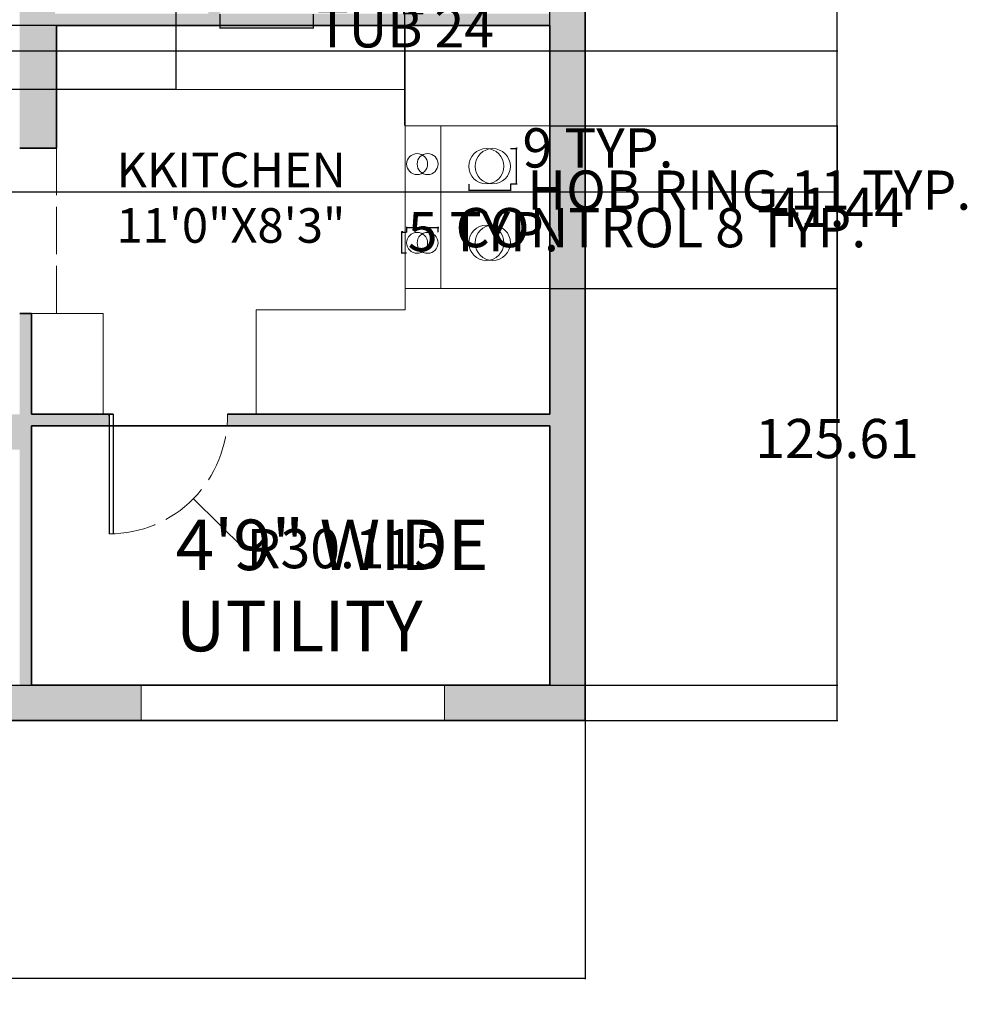
# Model space of a CAD drawing. Units: inches. Extents: x 300 to 1007, y 2 to 1069.
# Tile 6 of 12: x 766 to 1007, y 2 to 253. Entities that reach past the tile are written whole.
import ezdxf

# ---------------------------------------------------------------- set-up
doc = ezdxf.new("R2010")
doc.units = ezdxf.units.IN
doc.header["$MEASUREMENT"] = 0
doc.linetypes.add('ACAD_ISO02W100', pattern=[15, 12, -3])
for name, color, linetype, lineweight in [('A-ANNO-DIMS', 2, 'Continuous', 18), ('A-AREA-IDEN', 7, 'Continuous', 18), ('A-CASE', 8, 'Continuous', 18), ('A-DOOR', 3, 'Continuous', 25), ('A-DOOR-SWNG', 3, 'ACAD_ISO02W100', 13), ('A-EQPM', 9, 'Continuous', 18), ('A-GLAZ', 4, 'Continuous', 18), ('A-WALL', 7, 'Continuous', 35), ('A-WALL-OVHD', 8, 'ACAD_ISO02W100', 18)]:
    doc.layers.add(name, color=color, linetype=linetype, lineweight=lineweight)
doc.layers.add('A-WALL-PATT', color=9, linetype='Continuous', lineweight=9, true_color=0xc7c8ca)
doc.styles.get("Standard").update_dxf_attribs({"font": 'arial.ttf'})
doc.dimstyles.get("Standard").update_dxf_attribs({"dimtxt": 10, "dimasz": 0.18, "dimexe": 0.18, "dimexo": 0.0625, "dimgap": 0.09, "dimtad": 0, "dimtih": 1, "dimtoh": 1, "dimdec": 0, "dimzin": 0, "dimdsep": 46, "dimlunit": 3, "dimtxsty": 'Standard', "dimcen": 0.09, "dimadec": 0, "dimazin": 0, "dimtfac": 1, "dimtdec": 0, "dimtofl": 0, "dimtmove": 0, "dimatfit": 3, "dimfxl": 1, "dimtolj": 1, "dimtzin": 0, "dimarcsym": 0})

# ---------------------------------------------------------------- blocks, each defined once
blk = doc.blocks.new('COOKTOP-RING-9')
for centre in [(0, 0), (1.63, 0)]:
    blk.add_circle(centre, 4.49)
blk = doc.blocks.new('COOKTOP-CONTROL-5')
for centre in [(0, 0), (2.67, 0)]:
    blk.add_circle(centre, 2.67)
blk = doc.blocks.new('*D31')
at = {"layer": 'A-ANNO-DIMS', "color": 0, "lineweight": -2, "transparency": 16777216}
for p, q in [((868.84, 287.43), (863.76, 287.43)), ((863.94, 287.25), (863.94, 276.17)), ((863.94, 254.56), (863.94, 265.64)), ((868.84, 254.38), (863.76, 254.38))]:
    blk.add_line(p, q, dxfattribs=at)
at = {"layer": 'A-ANNO-DIMS', "color": 0, "transparency": 16777216}
for points in [[(863.91, 287.25), (863.97, 287.25), (863.94, 287.43)], [(863.91, 254.56), (863.97, 254.56), (863.94, 254.38)]]:
    blk.add_solid(points, dxfattribs=at)
at = {"layer": 'Defpoints', "color": 0, "transparency": 16777216}
for p in [(868.9, 287.43), (863.94, 254.38), (868.9, 254.38)]:
    blk.add_point(p, dxfattribs=at)
at = {"layer": 'A-ANNO-DIMS', "color": 0, "transparency": 16777216, "insert": (863.94, 270.91), "char_height": 10, "attachment_point": 5}
blk.add_mtext('\\A1;WC 33 TYP.', dxfattribs=at)
blk = doc.blocks.new('*D37')
at = {"layer": 'A-ANNO-DIMS', "color": 0, "lineweight": -2, "transparency": 16777216}
for p, q in [((817.12, 254.32), (817.12, 250.64)), ((840.87, 254.32), (840.87, 250.64)), ((817.3, 250.82), (840.69, 250.82)), ((840.87, 250.82), (841.05, 250.82))]:
    blk.add_line(p, q, dxfattribs=at)
at = {"layer": 'A-ANNO-DIMS', "color": 0, "transparency": 16777216}
for points in [[(817.3, 250.85), (817.3, 250.79), (817.12, 250.82)], [(840.69, 250.85), (840.69, 250.79), (840.87, 250.82)]]:
    blk.add_solid(points, dxfattribs=at)
at = {"layer": 'Defpoints', "color": 0, "transparency": 16777216}
for p in [(817.12, 254.38), (840.87, 254.38), (840.87, 250.82)]:
    blk.add_point(p, dxfattribs=at)
at = {"layer": 'A-ANNO-DIMS', "color": 0, "transparency": 16777216, "insert": (864.32, 250.82), "char_height": 10, "attachment_point": 5}
blk.add_mtext('\\A1;TUB 24', dxfattribs=at)
blk = doc.blocks.new('*D67')
at = {"layer": 'A-ANNO-DIMS', "color": 0, "lineweight": -2, "transparency": 16777216}
for p, q in [((880.48, 211), (880.48, 209.29)), ((891.09, 211), (891.09, 209.29)), ((880.66, 209.47), (890.91, 209.47)), ((891.09, 209.47), (891.27, 209.47))]:
    blk.add_line(p, q, dxfattribs=at)
at = {"layer": 'A-ANNO-DIMS', "color": 0, "transparency": 16777216}
for points in [[(880.66, 209.5), (880.66, 209.44), (880.48, 209.47)], [(890.91, 209.5), (890.91, 209.44), (891.09, 209.47)]]:
    blk.add_solid(points, dxfattribs=at)
at = {"layer": 'Defpoints', "color": 0, "transparency": 16777216}
for p in [(880.48, 211.06), (891.09, 211.06), (891.09, 209.47)]:
    blk.add_point(p, dxfattribs=at)
at = {"layer": 'A-ANNO-DIMS', "color": 0, "transparency": 16777216, "insert": (951.91, 209.47), "char_height": 10, "attachment_point": 5}
blk.add_mtext('\\A1;HOB RING 11 TYP.', dxfattribs=at)
blk = doc.blocks.new('*D68')
at = {"layer": 'A-ANNO-DIMS', "color": 0, "lineweight": -2, "transparency": 16777216}
for p, q in [((891.15, 220.04), (892.86, 220.04)), ((892.68, 220.04), (892.68, 220.22)), ((892.68, 220.22), (892.86, 220.22)), ((892.68, 211.24), (892.68, 219.86)), ((891.15, 211.06), (892.86, 211.06))]:
    blk.add_line(p, q, dxfattribs=at)
at = {"layer": 'A-ANNO-DIMS', "color": 0, "transparency": 16777216}
for points in [[(892.65, 219.86), (892.71, 219.86), (892.68, 220.04)], [(892.65, 211.24), (892.71, 211.24), (892.68, 211.06)]]:
    blk.add_solid(points, dxfattribs=at)
at = {"layer": 'Defpoints', "color": 0, "transparency": 16777216}
for p in [(891.09, 220.04), (892.68, 220.04), (891.09, 211.06)]:
    blk.add_point(p, dxfattribs=at)
at = {"layer": 'A-ANNO-DIMS', "color": 0, "transparency": 16777216, "insert": (913.4, 220.22), "char_height": 10, "attachment_point": 5}
blk.add_mtext('\\A1;9 TYP.', dxfattribs=at)
blk = doc.blocks.new('*D69')
at = {"layer": 'A-ANNO-DIMS', "color": 0, "lineweight": -2, "transparency": 16777216}
for p, q in [((864.68, 198.77), (864.68, 200.09)), ((864.86, 199.91), (872.49, 199.91)), ((872.67, 198.77), (872.67, 200.09)), ((872.67, 199.91), (872.85, 199.91))]:
    blk.add_line(p, q, dxfattribs=at)
at = {"layer": 'A-ANNO-DIMS', "color": 0, "transparency": 16777216}
for points in [[(864.86, 199.94), (864.86, 199.88), (864.68, 199.91)], [(872.49, 199.94), (872.49, 199.88), (872.67, 199.91)]]:
    blk.add_solid(points, dxfattribs=at)
at = {"layer": 'Defpoints', "color": 0, "transparency": 16777216}
for p in [(864.68, 198.71), (872.67, 199.91), (872.67, 198.71)]:
    blk.add_point(p, dxfattribs=at)
at = {"layer": 'A-ANNO-DIMS', "color": 0, "transparency": 16777216, "insert": (929.43, 199.91), "char_height": 10, "attachment_point": 5}
blk.add_mtext('\\A1;CONTROL 8 TYP.', dxfattribs=at)
blk = doc.blocks.new('*D70')
at = {"layer": 'A-ANNO-DIMS', "color": 0, "lineweight": -2, "transparency": 16777216}
for p, q in [((864.61, 198.71), (863.3, 198.71)), ((863.48, 198.71), (863.48, 198.89)), ((863.48, 198.89), (863.66, 198.89)), ((863.48, 193.56), (863.48, 198.53)), ((864.61, 193.38), (863.3, 193.38))]:
    blk.add_line(p, q, dxfattribs=at)
at = {"layer": 'A-ANNO-DIMS', "color": 0, "transparency": 16777216}
for points in [[(863.45, 198.53), (863.51, 198.53), (863.48, 198.71)], [(863.45, 193.56), (863.51, 193.56), (863.48, 193.38)]]:
    blk.add_solid(points, dxfattribs=at)
at = {"layer": 'Defpoints', "color": 0, "transparency": 16777216}
for p in [(863.48, 198.71), (864.68, 198.71), (864.68, 193.38)]:
    blk.add_point(p, dxfattribs=at)
at = {"layer": 'A-ANNO-DIMS', "color": 0, "transparency": 16777216, "insert": (884.2, 198.89), "char_height": 10, "attachment_point": 5}
blk.add_mtext('\\A1;5 TYP.', dxfattribs=at)
blk = doc.blocks.new('*D73')
at = {"layer": 'A-ANNO-DIMS', "color": 0, "lineweight": -2, "transparency": 16777216}
for p, q in [((420.12, 74.32), (420.12, 8.45)), ((910.12, 74.32), (910.12, 8.45)), ((420.3, 8.63), (653.8, 8.63)), ((909.94, 8.63), (676.44, 8.63))]:
    blk.add_line(p, q, dxfattribs=at)
at = {"layer": 'A-ANNO-DIMS', "color": 0, "transparency": 16777216}
for points in [[(420.3, 8.66), (420.3, 8.6), (420.12, 8.63)], [(909.94, 8.66), (909.94, 8.6), (910.12, 8.63)]]:
    blk.add_solid(points, dxfattribs=at)
at = {"layer": 'Defpoints', "color": 0, "transparency": 16777216}
for p in [(420.12, 74.38), (910.12, 74.38), (910.12, 8.63)]:
    blk.add_point(p, dxfattribs=at)
at = {"layer": 'A-ANNO-DIMS', "color": 0, "transparency": 16777216, "insert": (665.12, 8.63), "char_height": 10, "attachment_point": 5}
blk.add_mtext('\\A1;490', dxfattribs=at)
blk = doc.blocks.new('*D76')
at = {"layer": 'A-ANNO-DIMS', "color": 0, "lineweight": -2, "transparency": 16777216}
for p, q in [((910.18, 482.38), (974.48, 482.38)), ((974.3, 482.2), (974.3, 283.58)), ((974.3, 74.56), (974.3, 273.19)), ((910.18, 74.38), (974.48, 74.38))]:
    blk.add_line(p, q, dxfattribs=at)
at = {"layer": 'A-ANNO-DIMS', "color": 0, "transparency": 16777216}
for points in [[(974.27, 482.2), (974.33, 482.2), (974.3, 482.38)], [(974.27, 74.56), (974.33, 74.56), (974.3, 74.38)]]:
    blk.add_solid(points, dxfattribs=at)
at = {"layer": 'Defpoints', "color": 0, "transparency": 16777216}
for p in [(910.12, 482.38), (974.3, 482.38), (910.12, 74.38)]:
    blk.add_point(p, dxfattribs=at)
at = {"layer": 'A-ANNO-DIMS', "color": 0, "transparency": 16777216, "insert": (974.3, 278.38), "char_height": 10, "attachment_point": 5}
blk.add_mtext('\\A1;408', dxfattribs=at)
blk = doc.blocks.new('*D84')
at = {"layer": 'A-ANNO-DIMS', "color": 0, "lineweight": -2, "transparency": 16777216}
for p, q in [((864.25, 225.89), (864.25, 1063.03)), ((864.43, 1062.85), (865.73, 1062.85)), ((900.94, 1062.85), (899.65, 1062.85)), ((901.12, 225.89), (901.12, 1063.03))]:
    blk.add_line(p, q, dxfattribs=at)
at = {"layer": 'A-ANNO-DIMS', "color": 0, "transparency": 16777216}
for points in [[(864.43, 1062.88), (864.43, 1062.82), (864.25, 1062.85)], [(900.94, 1062.88), (900.94, 1062.82), (901.12, 1062.85)]]:
    blk.add_solid(points, dxfattribs=at)
at = {"layer": 'Defpoints', "color": 0, "transparency": 16777216}
for p in [(901.12, 1062.85), (864.25, 225.83), (901.12, 225.83)]:
    blk.add_point(p, dxfattribs=at)
at = {"layer": 'A-ANNO-DIMS', "color": 0, "transparency": 16777216, "insert": (882.69, 1062.85), "char_height": 10, "attachment_point": 5}
blk.add_mtext('\\A1;36.87', dxfattribs=at)
blk = doc.blocks.new('*D85')
at = {"layer": 'A-ANNO-DIMS', "color": 0, "lineweight": -2, "transparency": 16777216}
for p, q in [((901.18, 225.83), (974.48, 225.83)), ((974.3, 225.65), (974.3, 210.22)), ((974.3, 184.56), (974.3, 199.99)), ((901.18, 184.38), (974.48, 184.38))]:
    blk.add_line(p, q, dxfattribs=at)
at = {"layer": 'A-ANNO-DIMS', "color": 0, "transparency": 16777216}
for points in [[(974.27, 225.65), (974.33, 225.65), (974.3, 225.83)], [(974.27, 184.56), (974.33, 184.56), (974.3, 184.38)]]:
    blk.add_solid(points, dxfattribs=at)
at = {"layer": 'Defpoints', "color": 0, "transparency": 16777216}
for p in [(901.12, 225.83), (974.3, 225.83), (901.12, 184.38)]:
    blk.add_point(p, dxfattribs=at)
at = {"layer": 'A-ANNO-DIMS', "color": 0, "transparency": 16777216, "insert": (974.3, 205.1), "char_height": 10, "attachment_point": 5}
blk.add_mtext('\\A1;41.44', dxfattribs=at)
blk = doc.blocks.new('*D86')
at = {"layer": 'A-ANNO-DIMS', "color": 0, "lineweight": -2, "transparency": 16777216}
for p, q in [((805.95, 235.15), (805.95, 1063.03)), ((806.13, 1062.85), (822.02, 1062.85)), ((864.07, 1062.85), (848.18, 1062.85)), ((864.25, 235.15), (864.25, 1063.03))]:
    blk.add_line(p, q, dxfattribs=at)
at = {"layer": 'A-ANNO-DIMS', "color": 0, "transparency": 16777216}
for points in [[(806.13, 1062.88), (806.13, 1062.82), (805.95, 1062.85)], [(864.07, 1062.88), (864.07, 1062.82), (864.25, 1062.85)]]:
    blk.add_solid(points, dxfattribs=at)
at = {"layer": 'Defpoints', "color": 0, "transparency": 16777216}
for p in [(864.25, 1062.85), (805.95, 235.08), (864.25, 235.08)]:
    blk.add_point(p, dxfattribs=at)
at = {"layer": 'A-ANNO-DIMS', "color": 0, "transparency": 16777216, "insert": (835.1, 1062.85), "char_height": 10, "attachment_point": 5}
blk.add_mtext('\\A1;58.3', dxfattribs=at)
blk = doc.blocks.new('*D87')
at = {"layer": 'A-ANNO-DIMS', "color": 0, "lineweight": -2, "transparency": 16777216}
for p, q in [((805.89, 251.38), (354.19, 251.38)), ((354.37, 251.2), (354.37, 248.43)), ((354.37, 235.26), (354.37, 238.03)), ((805.89, 235.08), (354.19, 235.08))]:
    blk.add_line(p, q, dxfattribs=at)
at = {"layer": 'A-ANNO-DIMS', "color": 0, "transparency": 16777216}
for points in [[(354.34, 251.2), (354.4, 251.2), (354.37, 251.38)], [(354.34, 235.26), (354.4, 235.26), (354.37, 235.08)]]:
    blk.add_solid(points, dxfattribs=at)
at = {"layer": 'Defpoints', "color": 0, "transparency": 16777216}
for p in [(805.95, 251.38), (354.37, 235.08), (805.95, 235.08)]:
    blk.add_point(p, dxfattribs=at)
at = {"layer": 'A-ANNO-DIMS', "color": 0, "transparency": 16777216, "insert": (354.37, 243.23), "char_height": 10, "attachment_point": 5}
blk.add_mtext('\\A1;16.3', dxfattribs=at)
blk = doc.blocks.new('*D90')
at = {"layer": 'A-ANNO-DIMS', "color": 0, "lineweight": -2, "transparency": 16777216}
for p, q in [((429.18, 209), (974.48, 209)), ((974.3, 208.82), (974.3, 151.39)), ((974.3, 83.56), (974.3, 141)), ((429.18, 83.38), (974.48, 83.38))]:
    blk.add_line(p, q, dxfattribs=at)
at = {"layer": 'A-ANNO-DIMS', "color": 0, "transparency": 16777216}
for points in [[(974.27, 208.82), (974.33, 208.82), (974.3, 209)], [(974.27, 83.56), (974.33, 83.56), (974.3, 83.38)]]:
    blk.add_solid(points, dxfattribs=at)
at = {"layer": 'Defpoints', "color": 0, "transparency": 16777216}
for p in [(429.12, 209), (974.3, 209), (429.12, 83.38)]:
    blk.add_point(p, dxfattribs=at)
at = {"layer": 'A-ANNO-DIMS', "color": 0, "transparency": 16777216, "insert": (974.3, 146.19), "char_height": 10, "attachment_point": 5}
blk.add_mtext('\\A1;125.61', dxfattribs=at)
blk = doc.blocks.new('*D91')
at = {"layer": 'A-ANNO-DIMS', "color": 0, "lineweight": -2, "transparency": 16777216}
for p, q in [((429.18, 325.09), (974.48, 325.09)), ((974.3, 324.91), (974.3, 290.23)), ((974.3, 245.16), (974.3, 279.84)), ((429.18, 244.98), (974.48, 244.98))]:
    blk.add_line(p, q, dxfattribs=at)
at = {"layer": 'A-ANNO-DIMS', "color": 0, "transparency": 16777216}
for points in [[(974.27, 324.91), (974.33, 324.91), (974.3, 325.09)], [(974.27, 245.16), (974.33, 245.16), (974.3, 244.98)]]:
    blk.add_solid(points, dxfattribs=at)
at = {"layer": 'Defpoints', "color": 0, "transparency": 16777216}
for p in [(429.12, 325.09), (974.3, 325.09), (429.12, 244.98)]:
    blk.add_point(p, dxfattribs=at)
at = {"layer": 'A-ANNO-DIMS', "color": 0, "transparency": 16777216, "insert": (974.3, 285.04), "char_height": 10, "attachment_point": 5}
blk.add_mtext('\\A1;80.11', dxfattribs=at)
blk = doc.blocks.new('*D116')
at = {"layer": 'A-ANNO-DIMS', "color": 0, "lineweight": -2, "transparency": 16777216}
for p, q in [((788.82, 152.02), (789, 152.02)), ((788.91, 151.93), (788.91, 152.11)), ((823.19, 118.15), (810.46, 130.73)), ((823.37, 118.15), (823.19, 118.15))]:
    blk.add_line(p, q, dxfattribs=at)
at = {"layer": 'A-ANNO-DIMS', "color": 0, "transparency": 16777216}
blk.add_solid([(810.49, 130.75), (810.44, 130.7), (810.34, 130.85)], dxfattribs=at)
at = {"layer": 'Defpoints', "color": 0, "transparency": 16777216}
for p in [(788.91, 152.02), (810.34, 130.85)]:
    blk.add_point(p, dxfattribs=at)
at = {"layer": 'A-ANNO-DIMS', "color": 0, "transparency": 16777216, "insert": (849.04, 118.15), "char_height": 10, "attachment_point": 5}
blk.add_mtext('\\A1;R30.115', dxfattribs=at)

msp = doc.modelspace()

# ---------------------------------------------------------------- hatches: boundary and pattern name
at = {"layer": 'A-WALL-PATT'}
h = msp.add_hatch(color=256, dxfattribs=at)
h.dxf.hatch_style = 1
h.paths.add_polyline_path([(546.104, 999.4468), (478.8267, 999.4468), (478.8267, 869.2798, -0.06322715), (487.8267, 868.1328), (487.8267, 990.4468), (546.104, 990.4468)])
h.paths.add_polyline_path([(630.4852, 999.4468), (582.106, 999.4468), (582.106, 990.4468), (613.8267, 990.4468), (613.8267, 867.4468), (622.8267, 867.4468), (622.8267, 990.4468), (630.4852, 990.4468)])
h.paths.add_polyline_path([(702.0883, 999.4468), (650.4653, 999.4468), (650.4653, 990.4468), (682.8267, 990.4468), (682.8267, 960.0824, -0.02530575), (685.8267, 960.0478), (685.8267, 990.4468), (702.0883, 990.4468)])
h.paths.add_polyline_path([(850.8267, 999.4468), (737.5888, 999.4468), (737.5888, 990.4468), (841.8267, 990.4468), (841.8267, 950.5685), (850.8267, 950.5685)])
h.paths.add_polyline_path([(685.8267, 930.4465), (682.8267, 930.4465), (682.8267, 888.4468), (682.8267, 867.4468), (685.8267, 867.4468), (697.4169, 867.4468), (697.4169, 870.4468), (685.8267, 870.4468), (685.8267, 888.4468)])
h.paths.add_polyline_path([(682.8267, 931.4465), (654.3436, 931.4465, 0.00843109), (654.3267, 930.4465), (682.8267, 930.4465)])
h.paths.add_polyline_path([(685.8267, 931.4465), (682.8267, 931.4465), (682.8267, 930.4465), (685.8267, 930.4465)])
h.paths.add_polyline_path([(682.8267, 888.4468), (622.8267, 888.4468), (622.8267, 885.4468), (682.8267, 885.4468)])
h.paths.add_polyline_path([(850.8267, 870.4468), (850.8267, 914.7851), (841.8267, 914.7851), (841.8267, 870.4468), (732.7101, 870.4468, -0.02120595), (732.8267, 867.4468), (779.8267, 867.4468), (779.8267, 749.4468), (782.8267, 749.4468), (788.8267, 749.4468), (788.8267, 861.4468), (841.8267, 861.4468), (841.8267, 749.4468), (850.8267, 749.4468)])
h.paths.add_polyline_path([(622.8267, 810.4468), (487.8267, 810.4468), (487.8267, 833.2626), (478.8267, 833.2626), (478.8267, 609.4468), (478.8267, 482.3847), (487.8267, 482.3847), (487.8267, 801.4468), (620.8267, 801.4468), (622.8267, 801.4468)])
h.paths.add_polyline_path([(680.8267, 729.4468), (620.8267, 729.4468), (620.8267, 765.8246, -0.02111352), (617.8267, 766.0562), (617.8267, 698.7303), (620.8267, 698.7303), (620.8267, 726.4468), (680.8267, 726.4468)])
h.paths.add_polyline_path([(620.8267, 668.8122, -0.02498293), (617.8267, 668.6448), (617.8267, 618.4468), (600.3357, 618.4468), (600.3357, 609.4468), (652.9929, 609.4468), (652.9929, 618.4468), (620.8267, 618.4468)])
h.paths.add_polyline_path([(552.3393, 618.4468), (487.8267, 618.4468), (487.8267, 609.4468), (552.3393, 609.4468)], flags=17)
h.paths.add_polyline_path([(694.5763, 618.4468), (683.8267, 618.4468), (683.8267, 726.4468), (683.8267, 749.4468), (680.8267, 749.4468), (680.8267, 740.4468), (680.8267, 726.4468), (680.8267, 618.4468), (674.1573, 618.4468), (674.1573, 609.4468), (680.8267, 609.4468), (694.5763, 609.4468)])
h.paths.add_polyline_path([(850.8267, 642.8902), (841.8267, 642.8902), (841.8267, 618.4468), (782.8267, 618.4468), (782.8267, 708.0513, -0.02308839), (779.8267, 707.9092), (779.8267, 618.4468), (730.1068, 618.4468), (730.1068, 609.4468), (779.8267, 609.4468), (841.8267, 609.4468), (841.8267, 482.3847), (850.8267, 482.3847)])
h.paths.add_polyline_path([(850.8267, 749.4468), (841.8267, 749.4468), (841.8267, 705.9119), (850.8267, 705.9119)])
h.paths.add_polyline_path([(841.8267, 749.4468), (782.8267, 749.4468), (779.8267, 749.4468), (761.9959, 749.4468), (761.9959, 740.4468), (779.8267, 740.4468), (812.3267, 740.4468), (841.8267, 740.4468)])
h.paths.add_polyline_path([(669.1457, 482.3847), (604.489, 482.3847), (604.489, 473.3847), (631.1217, 473.3847), (631.1217, 436.0244, -0.02504709), (634.1217, 436.1748), (634.1217, 436.4367), (634.1217, 473.3847), (669.1457, 473.3847)], flags=17)
h.paths.add_polyline_path([(580.5305, 482.3847), (571.1217, 482.3847), (541.0813, 482.3847), (541.0813, 473.3847), (562.1217, 473.3847), (562.1217, 326.3847), (571.1217, 326.3847), (571.1217, 362.3847), (631.1217, 362.3847), (631.1217, 326.3847), (706.9024, 326.3847, -0.02105388), (706.9999, 329.3847), (634.1217, 329.3847), (634.1217, 365.3847), (634.1217, 406.1748), (631.1217, 406.1748), (631.1217, 365.3847), (571.1217, 365.3847), (571.1217, 473.3847), (580.5305, 473.3847)])
h.paths.add_polyline_path([(493.4756, 482.3847), (420.1217, 482.3847), (420.1217, 445.3134), (429.1217, 445.3134), (429.1217, 473.3847), (493.4756, 473.3847)])
h.paths.add_polyline_path([(786.2236, 482.3847), (716.7793, 482.3847), (716.7793, 473.3847), (766.1217, 473.3847), (766.1217, 329.3847), (742.5583, 329.3847), (742.5583, 326.3847), (766.1217, 326.3847), (766.1217, 316.0647), (769.1217, 316.0647), (769.1217, 326.3847), (769.1217, 473.3847), (786.2236, 473.3847)])
h.paths.add_polyline_path([(910.1217, 482.3847), (822.7166, 482.3847), (822.7166, 473.3847), (901.1217, 473.3847), (901.1217, 402.5393), (910.1217, 402.5393)])
h.paths.add_polyline_path([(910.1217, 366.1034), (901.1217, 366.1034), (901.1217, 329.3847), (814.1217, 329.3847), (814.1217, 312.5176), (817.1217, 312.5176), (817.1217, 326.3847), (901.1217, 326.3847), (901.1217, 293.0319), (910.1217, 293.0319), (910.1217, 326.3847)])
h.paths.add_polyline_path([(910.1217, 268.9355), (901.1217, 268.9355), (901.1217, 254.3847), (817.1217, 254.3847), (817.1217, 290.5411, -0.03396715), (814.1217, 290.3847), (814.1217, 254.3847), (775.1217, 254.3847), (775.1217, 281.5164), (769.1217, 281.5164), (769.1217, 292.1577), (766.1217, 292.1577), (766.1217, 254.3847), (766.1217, 220.1938), (775.5079, 220.1938), (775.5079, 251.3847), (817.1217, 251.3847), (901.1217, 251.3847), (901.1217, 152.3847), (819.0246, 152.3847, -0.02493798), (818.9117, 149.3847), (901.1217, 149.3847), (901.1217, 92.3847), (901.1217, 83.3847), (874.3528, 83.3847), (874.3528, 74.3847), (910.1217, 74.3847), (910.1217, 92.3847), (910.1217, 149.3847)])
h.paths.add_polyline_path([(429.1217, 325.0924), (420.1217, 325.0924), (420.1217, 263.3847), (420.1217, 244.9834), (429.1217, 244.9834), (429.1217, 269.3847), (571.1217, 269.3847), (571.1217, 272.3847), (562.1217, 272.3847), (429.1217, 272.3847)])
h.paths.add_polyline_path([(429.1217, 208.998), (420.1217, 208.998), (420.1217, 74.3847), (496.7704, 74.3847), (496.7704, 83.3847), (429.1217, 83.3847)])
h.paths.add_polyline_path([(598.4322, 83.3847), (571.1217, 83.3847), (571.1217, 122.1171), (562.1217, 122.1171), (562.1217, 83.3847), (544.6031, 83.3847), (544.6031, 74.3847), (598.4322, 74.3847)])
h.paths.add_polyline_path([(797.0822, 83.3847), (769.1217, 83.3847), (769.1217, 149.3847), (788.9123, 149.3847), (788.9123, 152.3847), (769.1217, 152.3847), (769.1217, 178.0167), (766.1217, 178.0167), (766.1217, 152.3847), (735.3598, 152.3847), (735.3598, 143.3847), (766.1217, 143.3847), (766.1217, 83.3847), (634.1217, 83.3847), (634.1217, 143.3847), (659.7326, 143.3847), (659.7326, 152.3847), (634.1217, 152.3847), (634.1217, 194.3847), (571.1217, 194.3847), (571.1217, 233.7289, -0.06379947), (562.1217, 234.7942), (562.1217, 163.4485), (567.7403, 163.4485), (567.7403, 152.3847), (571.1217, 152.3847), (571.1217, 191.3847), (631.1217, 191.3847), (631.1217, 83.3847), (621.979, 83.3847), (621.979, 74.3847), (631.1217, 74.3847), (797.0822, 74.3847)])

# ---------------------------------------------------------------- linework, layer by layer
at = {"layer": 'A-CASE'}
for p, q in [((805.95, 251.3847), (805.95, 235.0834)), ((864.2528, 235.0834), (864.2528, 251.3847)), ((864.2528, 251.3847), (864.2528, 178.9925)), ((805.95, 235.0834), (864.2528, 235.0834)), ((864.2528, 178.9925), (826.3381, 178.9925)), ((826.3381, 178.9925), (826.3381, 152.3847)), ((769.1217, 178.0167), (787.3757, 178.0167)), ((787.3757, 178.0167), (787.3757, 152.3847))]:
    msp.add_line(p, q, dxfattribs=at)
at = {"layer": 'A-DOOR'}
for p, q in [((788.9123, 152.3847), (788.9123, 121.9017)), ((788.9123, 152.3847), (789.9123, 152.3847)), ((789.9123, 152.3847), (789.9123, 121.9017))]:
    msp.add_line(p, q, dxfattribs=at)
at = {"layer": 'A-DOOR-SWNG'}
msp.add_arc((788.9123, 152.0164), 30.1146, 270, 0.700833, dxfattribs=at)
at = {"layer": 'A-EQPM'}
msp.add_line((873.3949, 225.8264), (873.3949, 184.3835), dxfattribs=at)
msp.add_lwpolyline([(864.2528, 225.8264), (901.1217, 225.8264), (901.1217, 184.3835), (864.2528, 184.3835)], close=True, dxfattribs=at)
at = {"layer": 'A-GLAZ'}
for p, q in [((797.0822, 83.3847), (797.0822, 74.3847)), ((874.3528, 83.3847), (874.3528, 74.3847))]:
    msp.add_line(p, q, dxfattribs=at)
at = {"layer": 'A-WALL'}
for p, q in [((910.1217, 482.3847), (910.1217, 74.3847)), ((775.5079, 251.3847), (817.1217, 251.3847)), ((775.5079, 220.1938), (775.5079, 251.3847)), ((901.1217, 251.3847), (817.1217, 251.3847)), ((901.1217, 251.3847), (901.1217, 152.3847)), ((910.1217, 251.3847), (910.1217, 152.3847)), ((766.1217, 220.1938), (775.5079, 220.1938)), ((766.1217, 178.0167), (769.1217, 178.0167)), ((769.1217, 152.3847), (769.1217, 178.0167)), ((789.9123, 152.3847), (769.1217, 152.3847)), ((901.1217, 152.3847), (819.0246, 152.3847)), ((901.1217, 149.3847), (769.1217, 149.3847)), ((769.1217, 149.3847), (769.1217, 83.3847)), ((901.1217, 149.3847), (901.1217, 92.3847)), ((910.1217, 149.3847), (910.1217, 74.3847)), ((901.1217, 83.3847), (901.1217, 92.3847)), ((910.1217, 74.3847), (910.1217, 92.3847)), ((769.1217, 83.3847), (901.1217, 83.3847)), ((420.1217, 74.3847), (910.1217, 74.3847)), ((631.1217, 74.3847), (910.1217, 74.3847))]:
    msp.add_line(p, q, dxfattribs=at)
at = {"layer": 'A-WALL-OVHD'}
msp.add_line((775.5079, 220.1938), (775.5079, 178.0167), dxfattribs=at)

# ---------------------------------------------------------------- block references
at = {"layer": 'A-EQPM'}
for name, p in [('COOKTOP-CONTROL-5', (867.3423, 216.1052)), ('COOKTOP-RING-9', (884.9688, 215.5512)), ('COOKTOP-CONTROL-5', (867.3423, 196.0419)), ('COOKTOP-RING-9', (884.9688, 196.0491))]:
    msp.add_blockref(name, p, dxfattribs=at)

# ---------------------------------------------------------------- texts
at = {"layer": 'A-AREA-IDEN'}
for s, height, p in [('KKITCHEN', 8.80899, (790.754, 210.2162)), ('11\'0"X8\'3"', 8.80899, (790.754, 196.0653)), ('4\'9" WIDE', 12.87594, (805.8699, 112.6762)), ('UTILITY', 12.87594, (805.8699, 91.9921))]:
    msp.add_text(s, height=height, dxfattribs=at).set_placement(p)

# ---------------------------------------------------------------- dimensions: what is measured, and where the dimension line sits
at = {"layer": 'A-ANNO-DIMS'}
for base, p1, p2, override, picture, middle in [((864.2528, 1062.8469), (805.95, 235.0834), (864.2528, 235.0834), {"dimdec": 1, "dimlfac": 1, "dimrnd": 0, "dimzin": 0, "dimdsep": 46, "dimlunit": 2}, '*D86', (835.1014, 1062.8469)), ((901.1217, 1062.8469), (864.2528, 225.8264), (901.1217, 225.8264), {"dimdec": 2, "dimlfac": 1, "dimrnd": 0, "dimzin": 0, "dimdsep": 46, "dimlunit": 2}, '*D84', (882.6872, 1062.8469)), ((910.1217, 8.6288), (420.1217, 74.3847), (910.1217, 74.3847), {"dimdec": 0, "dimlfac": 1, "dimrnd": 0, "dimzin": 0, "dimdsep": 46, "dimlunit": 2}, '*D73', (665.1217, 8.6288))]:
    dim = msp.add_linear_dim(base=base, p1=p1, p2=p2, dimstyle='Standard', override=override, dxfattribs=at)
    dim.commit()
    dim.dimension.update_dxf_attribs({"geometry": picture, "text_midpoint": middle})
for base, p1, p2, override, picture, middle in [((974.3023, 482.3847), (910.1217, 74.3847), (910.1217, 482.3847), {"dimdec": 0, "dimlfac": 1, "dimrnd": 0, "dimzin": 0, "dimdsep": 46, "dimlunit": 2}, '*D76', (974.3023, 278.3847)), ((974.3023, 325.0924), (429.1217, 244.9834), (429.1217, 325.0924), {"dimdec": 2, "dimlfac": 1, "dimrnd": 0, "dimzin": 0, "dimdsep": 46, "dimlunit": 2}, '*D91', (974.3023, 285.0379)), ((354.3658, 235.0834), (805.95, 251.3847), (805.95, 235.0834), {"dimdec": 1, "dimlfac": 1, "dimrnd": 0, "dimzin": 0, "dimdsep": 46, "dimlunit": 2}, '*D87', (354.3658, 243.2341)), ((974.3023, 225.8264), (901.1217, 184.3835), (901.1217, 225.8264), {"dimdec": 2, "dimlfac": 1, "dimrnd": 0, "dimzin": 0, "dimdsep": 46, "dimlunit": 2}, '*D85', (974.3023, 205.105)), ((974.3023, 208.998), (429.1217, 83.3847), (429.1217, 208.998), {"dimdec": 2, "dimlfac": 1, "dimrnd": 0, "dimzin": 0, "dimdsep": 46, "dimlunit": 2}, '*D90', (974.3023, 146.1913))]:
    dim = msp.add_linear_dim(base=base, p1=p1, p2=p2, angle=90, dimstyle='Standard', override=override, dxfattribs=at)
    dim.commit()
    dim.dimension.update_dxf_attribs({"geometry": picture, "text_midpoint": middle})
for base, p1, p2, angle, text, picture, middle in [((863.9413, 254.3847), (868.8982, 287.431), (868.8982, 254.3847), 270, 'WC <> TYP.', '*D31', (863.9413, 270.9078)), ((892.6799, 220.0409), (891.0885, 211.0615), (891.0885, 220.0409), 90, '<> TYP.', '*D68', (913.4035, 220.2209)), ((863.477, 198.7077), (864.6765, 193.3762), (864.6765, 198.7077), 90, '<> TYP.', '*D70', (884.2006, 198.8877))]:
    dim = msp.add_linear_dim(base=base, p1=p1, p2=p2, angle=angle, text=text, dimstyle='Standard', override={"dimdec": 0, "dimlfac": 1, "dimrnd": 0, "dimzin": 0, "dimdsep": 46, "dimlunit": 2}, dxfattribs=at)
    dim.commit()
    dim.dimension.update_dxf_attribs({"geometry": picture, "text_midpoint": middle})
for base, p1, p2, text, picture, middle in [((840.8701, 250.8225), (817.1217, 254.3847), (840.8701, 254.3847), 'TUB <>', '*D37', (864.3188, 250.8225)), ((891.0885, 209.4701), (880.4792, 211.0615), (891.0885, 211.0615), 'HOB RING <> TYP.', '*D67', (951.9076, 209.4701)), ((872.6738, 199.9073), (864.6765, 198.7077), (872.6738, 198.7077), 'CONTROL <> TYP.', '*D69', (929.4308, 199.9073))]:
    dim = msp.add_linear_dim(base=base, p1=p1, p2=p2, text=text, dimstyle='Standard', override={"dimdec": 0, "dimlfac": 1, "dimrnd": 0, "dimzin": 0, "dimdsep": 46, "dimlunit": 2}, dxfattribs=at)
    dim.commit()
    dim.dimension.update_dxf_attribs({"geometry": picture, "text_midpoint": middle})
dim = msp.add_radius_dim(center=(788.9123, 152.0164), mpoint=(810.3363, 130.8527), dimstyle='Standard', override={"dimdec": 3, "dimlfac": 1, "dimrnd": 0, "dimzin": 0, "dimdsep": 46, "dimlunit": 2}, dxfattribs=at)
dim.commit()
dim.dimension.update_dxf_attribs({"geometry": '*D116', "text_midpoint": (849.0405, 118.1545), "dimtype": 164})

doc.saveas('drawing.dxf')
